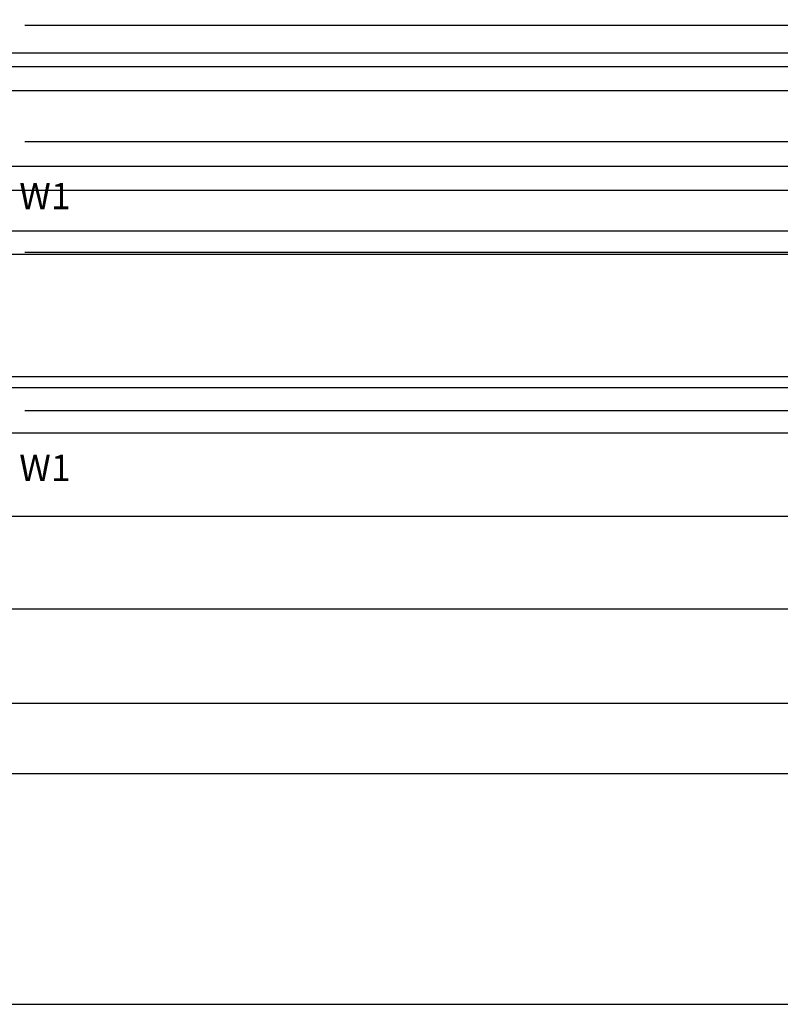
# Model space of a CAD drawing. Units: metres. Extents: x 2443.7 to 2482.9, y 2261.4 to 2287.
# Tile 6 of 8: x 2457.9 to 2466.1, y 2264.2 to 2274.8. Entities that reach past the tile are written whole.
import ezdxf

# ---------------------------------------------------------------- set-up
doc = ezdxf.new("R2010")
doc.units = ezdxf.units.M
for name, color, linetype, lineweight in [('A-ANNO-DIMS', 2, 'Continuous', 18), ('A-MODL', 7, 'Continuous', 25), ('text', 11, 'Continuous', 25)]:
    doc.layers.add(name, color=color, linetype=linetype, lineweight=lineweight)
doc.styles.get("Standard").update_dxf_attribs({"font": 'arial.ttf'})
doc.dimstyles.get("Standard").update_dxf_attribs({"dimtxt": 0.18, "dimasz": 0.18, "dimexe": 0.18, "dimexo": 0.0625, "dimgap": 0.09, "dimtad": 0, "dimtih": 1, "dimtoh": 1, "dimdec": 4, "dimzin": 0, "dimdsep": 46, "dimtxsty": 'Standard', "dimcen": 0.09, "dimadec": 0, "dimazin": 0, "dimtfac": 1, "dimtdec": 4, "dimtofl": 0, "dimtmove": 0, "dimatfit": 3, "dimfxl": 1, "dimtolj": 1, "dimtzin": 0, "dimarcsym": 0})

# ---------------------------------------------------------------- blocks, each defined once
blk = doc.blocks.new('aditya')
at = {"layer": 'text'}
for p in [(10.2, 7.908), (10.2, 4.965)]:
    blk.add_text('W1', height=0.2853, dxfattribs=at).set_placement(p)
blk = doc.blocks.new('*D23')
at = {"layer": 'A-ANNO-DIMS', "color": 0, "lineweight": -2, "transparency": 16777216}
for p, q in [((2457.945, 2274.76), (2482.243, 2274.76)), ((2482.063, 2274.58), (2482.063, 2269.642)), ((2482.063, 2264.34), (2482.063, 2269.278)), ((2453.645, 2264.16), (2482.243, 2264.16))]:
    blk.add_line(p, q, dxfattribs=at)
at = {"layer": 'A-ANNO-DIMS', "color": 0, "transparency": 16777216}
for points in [[(2482.033, 2274.58), (2482.093, 2274.58), (2482.063, 2274.76)], [(2482.033, 2264.34), (2482.093, 2264.34), (2482.063, 2264.16)]]:
    blk.add_solid(points, dxfattribs=at)
at = {"layer": 'Defpoints', "color": 0, "transparency": 16777216}
for p in [(2457.883, 2274.76), (2453.583, 2264.16), (2482.063, 2264.16)]:
    blk.add_point(p, dxfattribs=at)
at = {"layer": 'A-ANNO-DIMS', "color": 0, "transparency": 16777216, "insert": (2482.063, 2269.46), "char_height": 0.18, "attachment_point": 5}
blk.add_mtext('\\A1;10.6', dxfattribs=at)
blk = doc.blocks.new('*D34')
at = {"layer": 'A-ANNO-DIMS', "color": 0, "lineweight": -2, "transparency": 16777216}
for p, q in [((2457.945, 2274.76), (2482.243, 2274.76)), ((2482.063, 2274.58), (2482.063, 2274.313)), ((2482.063, 2273.682), (2482.063, 2273.949)), ((2457.945, 2273.502), (2482.243, 2273.502))]:
    blk.add_line(p, q, dxfattribs=at)
at = {"layer": 'A-ANNO-DIMS', "color": 0, "transparency": 16777216}
for points in [[(2482.033, 2274.58), (2482.093, 2274.58), (2482.063, 2274.76)], [(2482.033, 2273.682), (2482.093, 2273.682), (2482.063, 2273.502)]]:
    blk.add_solid(points, dxfattribs=at)
at = {"layer": 'Defpoints', "color": 0, "transparency": 16777216}
for p in [(2457.883, 2274.76), (2457.883, 2273.502), (2482.063, 2273.502)]:
    blk.add_point(p, dxfattribs=at)
at = {"layer": 'A-ANNO-DIMS', "color": 0, "transparency": 16777216, "insert": (2482.063, 2274.131), "char_height": 0.18, "attachment_point": 5}
blk.add_mtext('\\A1;1.258', dxfattribs=at)
blk = doc.blocks.new('*D35')
at = {"layer": 'A-ANNO-DIMS', "color": 0, "lineweight": -2, "transparency": 16777216}
for p, q in [((2457.945, 2272.302), (2482.243, 2272.302)), ((2482.063, 2272.122), (2482.063, 2271.625)), ((2482.063, 2270.767), (2482.063, 2271.264)), ((2457.945, 2270.587), (2482.243, 2270.587))]:
    blk.add_line(p, q, dxfattribs=at)
at = {"layer": 'A-ANNO-DIMS', "color": 0, "transparency": 16777216}
for points in [[(2482.033, 2272.122), (2482.093, 2272.122), (2482.063, 2272.302)], [(2482.033, 2270.767), (2482.093, 2270.767), (2482.063, 2270.587)]]:
    blk.add_solid(points, dxfattribs=at)
at = {"layer": 'Defpoints', "color": 0, "transparency": 16777216}
for p in [(2457.883, 2272.302), (2457.883, 2270.587), (2482.063, 2270.587)]:
    blk.add_point(p, dxfattribs=at)
at = {"layer": 'A-ANNO-DIMS', "color": 0, "transparency": 16777216, "insert": (2482.063, 2271.444), "char_height": 0.18, "attachment_point": 5}
blk.add_mtext('\\A1;1.71', dxfattribs=at)
blk = doc.blocks.new('*D37')
at = {"layer": 'A-ANNO-DIMS', "color": 0, "lineweight": -2, "transparency": 16777216}
for p, q in [((2450.187, 2274.312), (2482.243, 2274.312)), ((2482.063, 2274.132), (2482.063, 2273.478)), ((2482.063, 2272.46), (2482.063, 2273.114)), ((2450.187, 2272.28), (2482.243, 2272.28))]:
    blk.add_line(p, q, dxfattribs=at)
at = {"layer": 'A-ANNO-DIMS', "color": 0, "transparency": 16777216}
for points in [[(2482.033, 2274.132), (2482.093, 2274.132), (2482.063, 2274.312)], [(2482.033, 2272.46), (2482.093, 2272.46), (2482.063, 2272.28)]]:
    blk.add_solid(points, dxfattribs=at)
at = {"layer": 'Defpoints', "color": 0, "transparency": 16777216}
for p in [(2450.125, 2274.312), (2482.063, 2274.312), (2450.125, 2272.28)]:
    blk.add_point(p, dxfattribs=at)
at = {"layer": 'A-ANNO-DIMS', "color": 0, "transparency": 16777216, "insert": (2482.063, 2273.296), "char_height": 0.18, "attachment_point": 5}
blk.add_mtext('\\A1;2.032', dxfattribs=at)
blk = doc.blocks.new('*D40')
at = {"layer": 'A-ANNO-DIMS', "color": 0, "lineweight": -2, "transparency": 16777216}
for p, q in [((2456.575, 2272.973), (2482.243, 2272.973)), ((2482.063, 2272.793), (2482.063, 2272.088)), ((2482.063, 2271.019), (2482.063, 2271.724)), ((2456.575, 2270.839), (2482.243, 2270.839))]:
    blk.add_line(p, q, dxfattribs=at)
at = {"layer": 'A-ANNO-DIMS', "color": 0, "transparency": 16777216}
for points in [[(2482.033, 2272.793), (2482.093, 2272.793), (2482.063, 2272.973)], [(2482.033, 2271.019), (2482.093, 2271.019), (2482.063, 2270.839)]]:
    blk.add_solid(points, dxfattribs=at)
at = {"layer": 'Defpoints', "color": 0, "transparency": 16777216}
for p in [(2456.513, 2272.973), (2482.063, 2272.973), (2456.513, 2270.839)]:
    blk.add_point(p, dxfattribs=at)
at = {"layer": 'A-ANNO-DIMS', "color": 0, "transparency": 16777216, "insert": (2482.063, 2271.906), "char_height": 0.18, "attachment_point": 5}
blk.add_mtext('\\A1;2.13', dxfattribs=at)
blk = doc.blocks.new('*D47')
at = {"layer": 'A-ANNO-DIMS', "color": 0, "lineweight": -2, "transparency": 16777216}
for p, q in [((2482.063, 2267.42), (2482.063, 2267.6)), ((2482.063, 2267.6), (2482.243, 2267.6)), ((2448.968, 2267.42), (2482.243, 2267.42)), ((2482.063, 2266.838), (2482.063, 2267.24)), ((2448.968, 2266.658), (2482.243, 2266.658))]:
    blk.add_line(p, q, dxfattribs=at)
at = {"layer": 'A-ANNO-DIMS', "color": 0, "transparency": 16777216}
for points in [[(2482.033, 2267.24), (2482.093, 2267.24), (2482.063, 2267.42)], [(2482.033, 2266.838), (2482.093, 2266.838), (2482.063, 2266.658)]]:
    blk.add_solid(points, dxfattribs=at)
at = {"layer": 'Defpoints', "color": 0, "transparency": 16777216}
for p in [(2448.906, 2267.42), (2482.063, 2267.42), (2448.906, 2266.658)]:
    blk.add_point(p, dxfattribs=at)
at = {"layer": 'A-ANNO-DIMS', "color": 0, "transparency": 16777216, "insert": (2482.636, 2267.6), "char_height": 0.18, "attachment_point": 5}
blk.add_mtext('\\A1;0.762', dxfattribs=at)
blk = doc.blocks.new('*D49')
at = {"layer": 'A-ANNO-DIMS', "color": 0, "lineweight": -2, "transparency": 16777216}
for p, q in [((2448.386, 2269.444), (2482.243, 2269.444)), ((2482.063, 2269.264), (2482.063, 2269.125)), ((2482.063, 2268.622), (2482.063, 2268.761)), ((2448.386, 2268.442), (2482.243, 2268.442))]:
    blk.add_line(p, q, dxfattribs=at)
at = {"layer": 'A-ANNO-DIMS', "color": 0, "transparency": 16777216}
for points in [[(2482.033, 2269.264), (2482.093, 2269.264), (2482.063, 2269.444)], [(2482.033, 2268.622), (2482.093, 2268.622), (2482.063, 2268.442)]]:
    blk.add_solid(points, dxfattribs=at)
at = {"layer": 'Defpoints', "color": 0, "transparency": 16777216}
for p in [(2448.324, 2269.444), (2482.063, 2269.444), (2448.324, 2268.442)]:
    blk.add_point(p, dxfattribs=at)
at = {"layer": 'A-ANNO-DIMS', "color": 0, "transparency": 16777216, "insert": (2482.063, 2268.943), "char_height": 0.18, "attachment_point": 5}
blk.add_mtext('\\A1;1.00', dxfattribs=at)
blk = doc.blocks.new('*D54')
at = {"layer": 'A-ANNO-DIMS', "color": 0, "lineweight": -2, "transparency": 16777216}
for p, q in [((2482.063, 2273.233), (2482.063, 2273.413)), ((2482.063, 2273.413), (2482.243, 2273.413)), ((2452.54, 2273.233), (2482.243, 2273.233)), ((2482.063, 2272.713), (2482.063, 2273.053)), ((2452.54, 2272.533), (2482.243, 2272.533))]:
    blk.add_line(p, q, dxfattribs=at)
at = {"layer": 'A-ANNO-DIMS', "color": 0, "transparency": 16777216}
for points in [[(2482.033, 2273.053), (2482.093, 2273.053), (2482.063, 2273.233)], [(2482.033, 2272.713), (2482.093, 2272.713), (2482.063, 2272.533)]]:
    blk.add_solid(points, dxfattribs=at)
at = {"layer": 'Defpoints', "color": 0, "transparency": 16777216}
for p in [(2452.478, 2273.233), (2482.063, 2273.233), (2452.478, 2272.533)]:
    blk.add_point(p, dxfattribs=at)
at = {"layer": 'A-ANNO-DIMS', "color": 0, "transparency": 16777216, "insert": (2482.497, 2273.413), "char_height": 0.18, "attachment_point": 5}
blk.add_mtext('\\A1;0.7', dxfattribs=at)
blk = doc.blocks.new('*D56')
at = {"layer": 'A-ANNO-DIMS', "color": 0, "lineweight": -2, "transparency": 16777216}
for p, q in [((2482.062768, 2274.639673), (2482.062768, 2274.819673)), ((2453.208999, 2274.459673), (2482.242768, 2274.459673)), ((2453.07969, 2274.053273), (2482.242768, 2274.053273)), ((2482.062768, 2273.873273), (2482.062768, 2273.693273))]:
    blk.add_line(p, q, dxfattribs=at)
at = {"layer": 'A-ANNO-DIMS', "color": 0, "transparency": 16777216}
for points in [[(2482.032768, 2274.639673), (2482.092768, 2274.639673), (2482.062768, 2274.459673)], [(2482.032768, 2273.873273), (2482.092768, 2273.873273), (2482.062768, 2274.053273)]]:
    blk.add_solid(points, dxfattribs=at)
at = {"layer": 'Defpoints', "color": 0, "transparency": 16777216}
for p in [(2453.146499, 2274.459673), (2482.062768, 2274.459673), (2453.01719, 2274.053273)]:
    blk.add_point(p, dxfattribs=at)
at = {"layer": 'A-ANNO-DIMS', "color": 0, "transparency": 16777216, "insert": (2482.062768, 2274.256473), "char_height": 0.18, "attachment_point": 5}
blk.add_mtext('\\A1;0.41', dxfattribs=at)
blk = doc.blocks.new('*D58')
at = {"layer": 'A-ANNO-DIMS', "color": 0, "lineweight": -2, "transparency": 16777216}
for p, q in [((2448.715, 2270.958), (2482.243, 2270.958)), ((2482.063, 2270.778), (2482.063, 2270.527)), ((2448.728, 2270.347), (2482.243, 2270.347)), ((2482.063, 2270.347), (2482.063, 2270.167)), ((2482.063, 2270.167), (2481.883, 2270.167))]:
    blk.add_line(p, q, dxfattribs=at)
at = {"layer": 'A-ANNO-DIMS', "color": 0, "transparency": 16777216}
for points in [[(2482.033, 2270.778), (2482.093, 2270.778), (2482.063, 2270.958)], [(2482.033, 2270.527), (2482.093, 2270.527), (2482.063, 2270.347)]]:
    blk.add_solid(points, dxfattribs=at)
at = {"layer": 'Defpoints', "color": 0, "transparency": 16777216}
for p in [(2448.653, 2270.958), (2448.665, 2270.347), (2482.063, 2270.347)]:
    blk.add_point(p, dxfattribs=at)
at = {"layer": 'A-ANNO-DIMS', "color": 0, "transparency": 16777216, "insert": (2481.576, 2270.167), "char_height": 0.18, "attachment_point": 5}
blk.add_mtext('\\A1;0.61', dxfattribs=at)

msp = doc.modelspace()

# ---------------------------------------------------------------- block references
at = {"layer": 'A-MODL'}
msp.add_blockref('aditya', (2447.682762, 2264.859673), dxfattribs=at)

# ---------------------------------------------------------------- dimensions: what is measured, and where the dimension line sits
at = {"layer": 'A-ANNO-DIMS'}
for base, p1, p2, override, picture, middle in [((2482.062768, 2274.459673), (2453.01719, 2274.053273), (2453.146499, 2274.459673), {"dimdec": 2, "dimlfac": 1, "dimrnd": 0, "dimzin": 0, "dimdsep": 46, "dimlunit": 2}, '*D56', (2482.062768, 2274.256473)), ((2482.062768, 2264.159673), (2457.882762, 2274.759673), (2453.582762, 2264.159673), {"dimdec": 1, "dimlfac": 1, "dimrnd": 0, "dimzin": 0, "dimdsep": 46, "dimlunit": 2}, '*D23', (2482.062768, 2269.459673)), ((2482.062768, 2273.501681), (2457.882762, 2274.759673), (2457.882762, 2273.501681), {"dimdec": 3, "dimlfac": 1, "dimrnd": 0, "dimzin": 0, "dimdsep": 46, "dimlunit": 2}, '*D34', (2482.062768, 2274.130677)), ((2482.062768, 2274.312339), (2450.124936, 2272.280339), (2450.124936, 2274.312339), {"dimdec": 3, "dimlfac": 1, "dimrnd": 0, "dimzin": 0, "dimdsep": 46, "dimlunit": 2}, '*D37', (2482.062768, 2273.296339)), ((2482.062768, 2273.233088), (2452.477762, 2272.533088), (2452.477762, 2273.233088), {"dimdec": 1, "dimlfac": 1, "dimrnd": 0, "dimzin": 0, "dimdsep": 46, "dimlunit": 2}, '*D54', (2482.496622, 2273.413088)), ((2482.062768, 2272.973048), (2456.512931, 2270.839448), (2456.512931, 2272.973048), {"dimdec": 2, "dimlfac": 1, "dimrnd": 0, "dimzin": 0, "dimdsep": 46, "dimlunit": 2}, '*D40', (2482.062768, 2271.906248)), ((2482.062768, 2270.586919), (2457.882762, 2272.301681), (2457.882762, 2270.586919), {"dimdec": 2, "dimlfac": 1, "dimrnd": 0, "dimzin": 0, "dimdsep": 46, "dimlunit": 2}, '*D35', (2482.062768, 2271.4443)), ((2482.062768, 2270.346637), (2448.652642, 2270.958301), (2448.665238, 2270.346637), {"dimdec": 2, "dimlfac": 1, "dimrnd": 0, "dimzin": 0, "dimdsep": 46, "dimlunit": 2}, '*D58', (2481.576363, 2270.166637)), ((2482.062768, 2269.444297), (2448.323976, 2268.442446), (2448.323976, 2269.444297), {"dimdec": 2, "dimlfac": 1, "dimrnd": 0, "dimzin": 0, "dimdsep": 46, "dimlunit": 2}, '*D49', (2482.062768, 2268.943372)), ((2482.062768, 2267.419676), (2448.905882, 2266.657676), (2448.905882, 2267.419676), {"dimdec": 3, "dimlfac": 1, "dimrnd": 0, "dimzin": 0, "dimdsep": 46, "dimlunit": 2}, '*D47', (2482.635551, 2267.599676))]:
    dim = msp.add_linear_dim(base=base, p1=p1, p2=p2, angle=90, dimstyle='Standard', override=override, dxfattribs=at)
    dim.commit()
    dim.dimension.update_dxf_attribs({"geometry": picture, "text_midpoint": middle})

doc.saveas('drawing.dxf')
